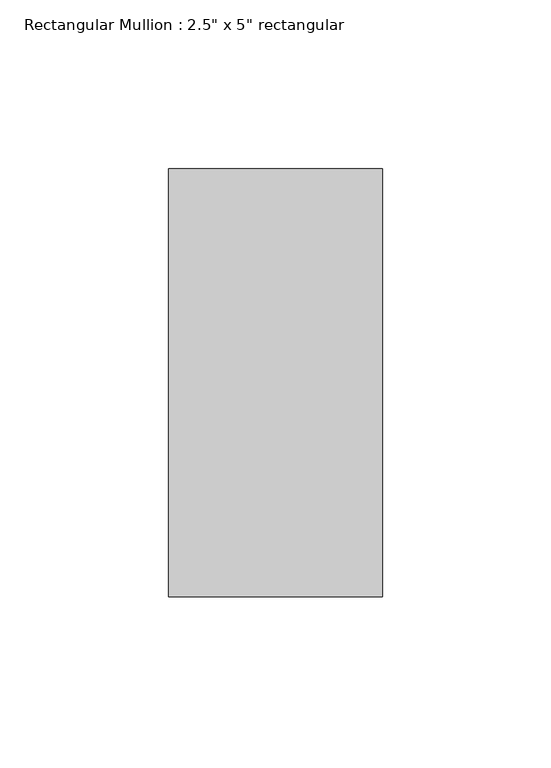
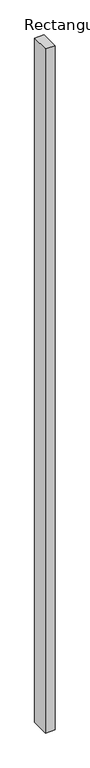
"""IFC4 building model written with IfcOpenShell, lengths in millimetres: member geometry."""

from ifc_helpers import new_model, si_unit, frame, origin, place, context, project, spatial, polyline, outline, extrude, source, transform, mapped, element, save


def member_8d537d56(model_context):
    return source(origin(), model_context, "Body", "SweptSolid", [
        extrude(outline(polyline([(0.0, 63.5), (0.0, -63.5), (-63.5, -63.5), (-63.5, 63.5), (0.0, 63.5)])), frame((0.0, 0.0, -4895.3171854), z_axis=(0.0, 0.0, 1.0), x_axis=(1.0, 0.0, 0.0)), (0.0, 0.0, 1.0), 4895.3171854),
    ])


if __name__ == "__main__":
    model = new_model("IFC4")
    model_context = context("Model", 3, world=origin())
    ifc_project = project(units=[si_unit("LENGTHUNIT", "METRE", prefix="MILLI")], contexts=[model_context])
    site = spatial("IfcSite", under=ifc_project)
    building = spatial("IfcBuilding", under=site)
    placement = place(None, origin())
    member_shape = member_8d537d56(model_context)
    element("IfcMember", 1, ObjectType="Rectangular Mullion : 2.5\" x 5\" rectangular", at=placement, inside=building, context=model_context, shape_type="MappedRepresentation", body=[
        mapped(member_shape, transform((0.0, 0.0, 0.0), x_axis=(1.0, 0.0, 0.0), y_axis=(0.0, 1.0, 0.0), z_axis=(0.0, 0.0, 1.0))),
    ])
    save(model, "model.ifc")

# Revit data of these elements
# Type "Rectangular Mullion : 2.5\" x 5\" rectangular"
#   built-in parameter 1007304 = 0.416667 (stored number, unit not read)
#   built-in parameter 1007301 = 0.104167 (stored number, unit not read)
#   built-in parameter 1007300 = 0.104167 (stored number, unit not read)
# Element 1 (IfcMember, "Rectangular Mullion : 2.5\" x 5\" rectangular")
#   Materials on its faces: "Aluminum"
# Materials
#   "Aluminum": class "Metal", colour RGB 247 247 247, transparency 0, Description = "Aluminum 6061", Cost = 0
